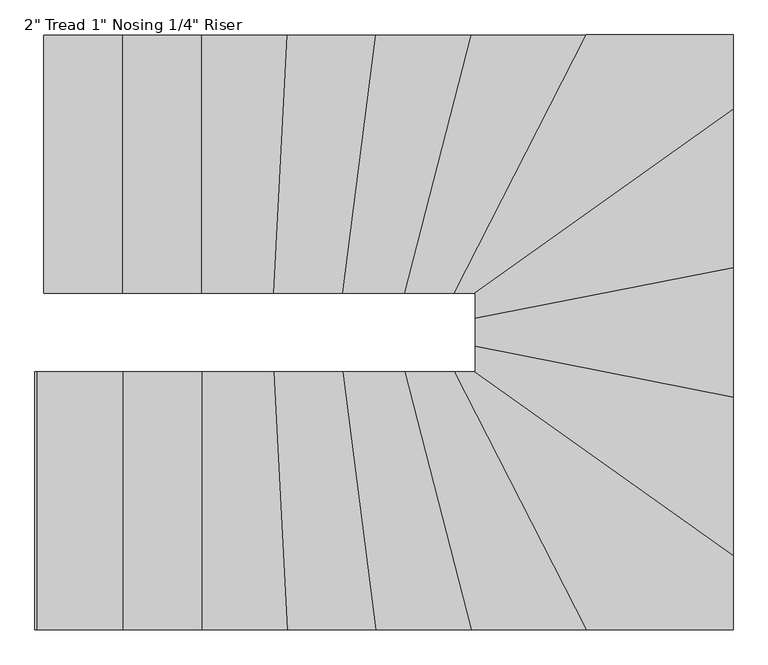
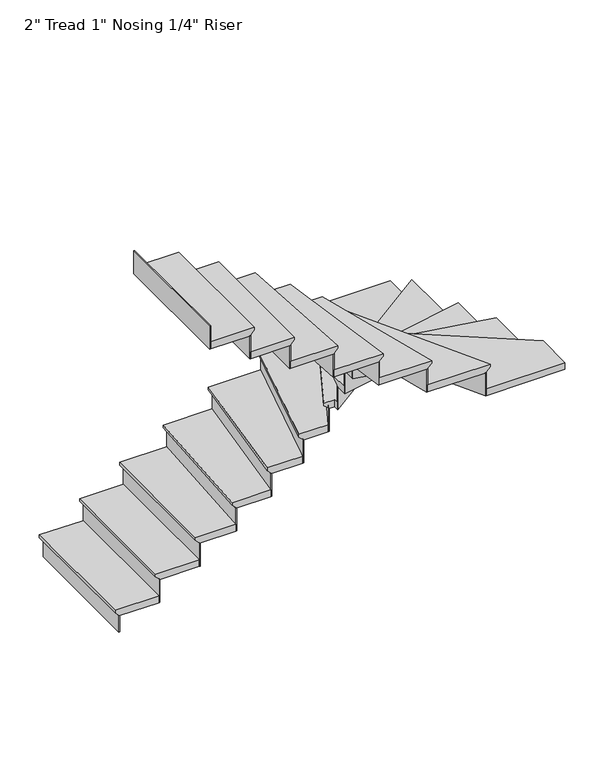
"""IFC4 building model written with IfcOpenShell, lengths in millimetres: stair flight geometry."""

from ifc_helpers import new_model, si_unit, origin, place, context, project, spatial, faceted_brep, source, transform, mapped, element, save


def stair_flight_9e462077(model_context):
    return source(origin(), model_context, "Body", "Brep", [
        faceted_brep([(1342.8282136, -2159.7365003, 9751.4833333), (1342.8282136, -2159.7365003, 9770.5333333), (1342.8282136, -1245.3365003, 9770.5333333), (1342.8282136, -1245.3365003, 9751.4833333), (1368.2282136, -2159.7365003, 9726.0833333), (1368.2282136, -1245.3365003, 9726.0833333), (1647.6282136, -2159.7365003, 9770.5333333), (1647.6282136, -1245.3365003, 9770.5333333), (1368.2282136, -1245.3365003, 9719.7333333), (1647.6282136, -1245.3365003, 9719.7333333), (1647.6282136, -2159.7365003, 9719.7333333), (1368.2282136, -2159.7365003, 9719.7333333)], [[[0, 1, 2, 3]], [[4, 0, 3, 5]], [[2, 1, 6, 7]], [[8, 9, 10, 11]], [[2, 7, 9, 8, 5, 3]], [[8, 11, 4, 5]], [[6, 1, 0, 4, 11, 10]], [[7, 6, 10, 9]]]),
        faceted_brep([(1368.2282136, -2159.7365003, 9719.7333333), (1368.2282136, -2159.7365003, 9601.2), (1374.5782136, -2159.7365003, 9601.2), (1374.5782136, -2159.7365003, 9719.7333333), (1368.2282136, -1245.3365003, 9719.7333333), (1374.5782136, -1245.3365003, 9719.7333333), (1374.5782136, -1245.3365003, 9601.2), (1368.2282136, -1245.3365003, 9601.2)], [[[0, 1, 2, 3]], [[4, 5, 6, 7]], [[1, 0, 4, 7]], [[2, 1, 7, 6]], [[3, 2, 6, 5]], [[0, 3, 5, 4]]]),
        faceted_brep([(1647.6282136, -2159.7365003, 9889.0666667), (1647.6282136, -2159.7365003, 9719.7333333), (1653.9782136, -2159.7365003, 9719.7333333), (1653.9782136, -2159.7365003, 9889.0666667), (1647.6282136, -1245.3365003, 9889.0666667), (1653.9782136, -1245.3365003, 9889.0666667), (1653.9782136, -1245.3365003, 9719.7333333), (1647.6282136, -1245.3365003, 9719.7333333)], [[[0, 1, 2, 3]], [[4, 5, 6, 7]], [[1, 0, 4, 7]], [[2, 1, 7, 6]], [[3, 2, 6, 5]], [[0, 3, 5, 4]]]),
        faceted_brep([(1622.2282136, -1245.3365003, 9939.8666667), (1622.2282136, -2159.7365003, 9939.8666667), (1927.0282136, -2159.7365003, 9939.8666667), (1927.0282136, -1245.3365003, 9939.8666667), (1647.6282136, -1245.3365003, 9889.0666667), (1927.0282136, -1245.3365003, 9889.0666667), (1927.0282136, -2159.7365003, 9889.0666667), (1647.6282136, -2159.7365003, 9889.0666667), (1647.6282136, -1245.3365003, 9895.4166667), (1622.2282136, -1245.3365003, 9920.8166667), (1647.6282136, -2159.7365003, 9895.4166667), (1622.2282136, -2159.7365003, 9920.8166667)], [[[0, 1, 2, 3]], [[4, 5, 6, 7]], [[0, 3, 5, 4, 8, 9]], [[4, 7, 10, 8]], [[2, 1, 11, 10, 7, 6]], [[3, 2, 6, 5]], [[11, 1, 0, 9]], [[10, 11, 9, 8]]]),
        faceted_brep([(1927.0282136, -2159.7365003, 10058.4), (1927.0282136, -2159.7365003, 9889.0666667), (1933.3782136, -2159.7365003, 9889.0666667), (1933.3782136, -2159.7365003, 10058.4), (1927.0282136, -1245.3365003, 10058.4), (1933.3782136, -1245.3365003, 10058.4), (1933.3782136, -1245.3365003, 9889.0666667), (1927.0282136, -1245.3365003, 9889.0666667)], [[[0, 1, 2, 3]], [[4, 5, 6, 7]], [[1, 0, 4, 7]], [[2, 1, 7, 6]], [[3, 2, 6, 5]], [[0, 3, 5, 4]]]),
        faceted_brep([(1901.6282136, -1245.3365003, 10109.2), (1901.6282136, -2159.7365003, 10109.2), (2182.6953751, -2159.7365003, 10109.2), (2230.2296455, -1245.3365003, 10109.2), (1927.0282136, -1245.3365003, 10058.4), (2230.2296455, -1245.3365003, 10058.4), (2182.6953751, -2159.7365003, 10058.4), (1927.0282136, -2159.7365003, 10058.4), (1927.0282136, -1245.3365003, 10064.75), (1901.6282136, -1245.3365003, 10090.15), (1927.0282136, -2159.7365003, 10064.75), (1901.6282136, -2159.7365003, 10090.15)], [[[0, 1, 2, 3]], [[4, 5, 6, 7]], [[0, 3, 5, 4, 8, 9]], [[4, 7, 10, 8]], [[2, 1, 11, 10, 7, 6]], [[3, 2, 6, 5]], [[11, 1, 0, 9]], [[10, 11, 9, 8]]]),
        faceted_brep([(2182.6953751, -2159.7365003, 10227.7333333), (2182.6953751, -2159.7365003, 10058.4), (2189.0539493, -2159.7365003, 10058.4), (2189.0539493, -2159.7365003, 10227.7333333), (2230.2296455, -1245.3365003, 10227.7333333), (2236.5882197, -1245.3365003, 10227.7333333), (2236.5882197, -1245.3365003, 10058.4), (2230.2296455, -1245.3365003, 10058.4)], [[[0, 1, 2, 3]], [[4, 5, 6, 7]], [[1, 0, 4, 7]], [[2, 1, 7, 6]], [[3, 2, 6, 5]], [[0, 3, 5, 4]]]),
        faceted_brep([(2204.7953488, -1245.3365003, 10278.5333333), (2157.2610784, -2159.7365003, 10278.5333333), (2426.8620749, -2159.7365003, 10278.5333333), (2545.2181266, -1245.3365003, 10278.5333333), (2230.2296455, -1245.3365003, 10227.7333333), (2545.2181266, -1245.3365003, 10227.7333333), (2426.8620749, -2159.7365003, 10227.7333333), (2182.6953751, -2159.7365003, 10227.7333333), (2230.2296455, -1245.3365003, 10234.0833333), (2204.7953488, -1245.3365003, 10259.4833333), (2182.6953751, -2159.7365003, 10234.0833333), (2157.2610784, -2159.7365003, 10259.4833333)], [[[0, 1, 2, 3]], [[4, 5, 6, 7]], [[0, 3, 5, 4, 8, 9]], [[4, 7, 10, 8]], [[2, 1, 11, 10, 7, 6]], [[3, 2, 6, 5]], [[11, 1, 0, 9]], [[10, 11, 9, 8]]]),
        faceted_brep([(2426.8620749, -2159.7365003, 10397.0666667), (2426.8620749, -2159.7365003, 10227.7333333), (2433.2650467, -2159.7365003, 10227.7333333), (2433.2650467, -2159.7365003, 10397.0666667), (2545.2181266, -1245.3365003, 10397.0666667), (2551.6210984, -1245.3365003, 10397.0666667), (2551.6210984, -1245.3365003, 10227.7333333), (2545.2181266, -1245.3365003, 10227.7333333)], [[[0, 1, 2, 3]], [[4, 5, 6, 7]], [[1, 0, 4, 7]], [[2, 1, 7, 6]], [[3, 2, 6, 5]], [[0, 3, 5, 4]]]),
        faceted_brep([(2519.6062395, -1245.3365003, 10447.8666667), (2401.2501878, -2159.7365003, 10447.8666667), (2648.4892974, -2159.7365003, 10447.8666667), (2883.6197448, -1245.3365003, 10447.8666667), (2545.2181266, -1245.3365003, 10397.0666667), (2883.6197448, -1245.3365003, 10397.0666667), (2648.4892974, -2159.7365003, 10397.0666667), (2426.8620749, -2159.7365003, 10397.0666667), (2545.2181266, -1245.3365003, 10403.4166667), (2519.6062395, -1245.3365003, 10428.8166667), (2426.8620749, -2159.7365003, 10403.4166667), (2401.2501878, -2159.7365003, 10428.8166667)], [[[0, 1, 2, 3]], [[4, 5, 6, 7]], [[0, 3, 5, 4, 8, 9]], [[4, 7, 10, 8]], [[2, 1, 11, 10, 7, 6]], [[3, 2, 6, 5]], [[11, 1, 0, 9]], [[10, 11, 9, 8]]]),
        faceted_brep([(2648.4892974, -2159.7365003, 10566.4), (2648.4892974, -2159.7365003, 10397.0666667), (2655.0458743, -2159.7365003, 10397.0666667), (2655.0458743, -2159.7365003, 10566.4), (2883.6197448, -1245.3365003, 10566.4), (2890.1763217, -1245.3365003, 10566.4), (2890.1763217, -1245.3365003, 10397.0666667), (2883.6197448, -1245.3365003, 10397.0666667)], [[[0, 1, 2, 3]], [[4, 5, 6, 7]], [[1, 0, 4, 7]], [[2, 1, 7, 6]], [[3, 2, 6, 5]], [[0, 3, 5, 4]]]),
        faceted_brep([(2857.3934373, -1245.3365003, 10617.2), (2622.2629899, -2159.7365003, 10617.2), (2824.8359335, -2159.7365003, 10617.2), (3293.6605548, -1245.3365003, 10617.2), (2883.6197448, -1245.3365003, 10566.4), (3293.6605548, -1245.3365003, 10566.4), (2824.8359335, -2159.7365003, 10566.4), (2648.4892974, -2159.7365003, 10566.4), (2883.6197448, -1245.3365003, 10572.75), (2857.3934373, -1245.3365003, 10598.15), (2648.4892974, -2159.7365003, 10572.75), (2622.2629899, -2159.7365003, 10598.15)], [[[0, 1, 2, 3]], [[4, 5, 6, 7]], [[0, 3, 5, 4, 8, 9]], [[4, 7, 10, 8]], [[2, 1, 11, 10, 7, 6]], [[3, 2, 6, 5]], [[11, 1, 0, 9]], [[10, 11, 9, 8]]]),
        faceted_brep([(2824.8359335, -2159.7365003, 10735.7333333), (2824.8359335, -2159.7365003, 10566.4), (2831.9719166, -2159.7365003, 10566.4), (2831.9719166, -2159.7365003, 10735.7333333), (3293.6605548, -1245.3365003, 10735.7333333), (3300.7965379, -1245.3365003, 10735.7333333), (3300.7965379, -1245.3365003, 10566.4), (3293.6605548, -1245.3365003, 10566.4)], [[[0, 1, 2, 3]], [[4, 5, 6, 7]], [[1, 0, 4, 7]], [[2, 1, 7, 6]], [[3, 2, 6, 5]], [[0, 3, 5, 4]]]),
        faceted_brep([(3784.9599055, -1539.017634, 10786.5333333), (3784.9599055, -1245.3365003, 10786.5333333), (3265.1166223, -1245.3365003, 10786.5333333), (2796.2920009, -2159.7365003, 10786.5333333), (2870.5599055, -2159.7365003, 10786.5333333), (2870.5599055, -2189.2915832, 10786.5333333), (3784.9599055, -1245.3365003, 10735.7333333), (3784.9599055, -1539.017634, 10735.7333333), (2870.5599055, -2189.2915832, 10735.7333333), (2870.5599055, -2159.7365003, 10735.7333333), (2824.8359335, -2159.7365003, 10735.7333333), (3293.6605548, -1245.3365003, 10735.7333333), (3293.6605548, -1245.3365003, 10742.0833333), (3265.1166223, -1245.3365003, 10767.4833333), (2824.8359335, -2159.7365003, 10742.0833333), (2796.2920009, -2159.7365003, 10767.4833333)], [[[0, 1, 2, 3, 4, 5]], [[6, 7, 8, 9, 10, 11]], [[1, 0, 7, 6]], [[2, 1, 6, 11, 12, 13]], [[11, 10, 14, 12]], [[4, 3, 15, 14, 10, 9]], [[5, 4, 9, 8]], [[0, 5, 8, 7]], [[15, 3, 2, 13]], [[14, 15, 13, 12]]]),
        faceted_brep([(2870.5599055, -2189.2915832, 10905.0666667), (2870.5599055, -2189.2915832, 10735.7333333), (2870.5599055, -2197.083558, 10735.7333333), (2870.5599055, -2197.083558, 10905.0666667), (3784.9599055, -1539.017634, 10905.0666667), (3784.9599055, -1546.8096088, 10905.0666667), (3784.9599055, -1546.8096088, 10735.7333333), (3784.9599055, -1539.017634, 10735.7333333)], [[[0, 1, 2, 3]], [[4, 5, 6, 7]], [[1, 0, 4, 7]], [[2, 1, 7, 6]], [[3, 2, 6, 5]], [[0, 3, 5, 4]]]),
        faceted_brep([(3784.9599055, -1507.8497349, 10955.8666667), (2870.5599055, -2158.123684, 10955.8666667), (2870.5599055, -2275.7456703, 10955.8666667), (3784.9599055, -2095.5048139, 10955.8666667), (3784.9599055, -1539.017634, 10905.0666667), (3784.9599055, -2095.5048139, 10905.0666667), (2870.5599055, -2275.7456703, 10905.0666667), (2870.5599055, -2189.2915832, 10905.0666667), (3784.9599055, -1539.017634, 10911.4166667), (3784.9599055, -1507.8497349, 10936.8166667), (2870.5599055, -2189.2915832, 10911.4166667), (2870.5599055, -2158.123684, 10936.8166667)], [[[0, 1, 2, 3]], [[4, 5, 6, 7]], [[0, 3, 5, 4, 8, 9]], [[4, 7, 10, 8]], [[2, 1, 11, 10, 7, 6]], [[3, 2, 6, 5]], [[11, 1, 0, 9]], [[10, 11, 9, 8]]]),
        faceted_brep([(2870.5599055, -2275.7456703, 11074.4), (2870.5599055, -2275.7456703, 10905.0666667), (2870.5599055, -2282.2178557, 10905.0666667), (2870.5599055, -2282.2178557, 11074.4), (3784.9599055, -2095.5048139, 11074.4), (3784.9599055, -2101.9769994, 11074.4), (3784.9599055, -2101.9769994, 10905.0666667), (3784.9599055, -2095.5048139, 10905.0666667)], [[[0, 1, 2, 3]], [[4, 5, 6, 7]], [[1, 0, 4, 7]], [[2, 1, 7, 6]], [[3, 2, 6, 5]], [[0, 3, 5, 4]]]),
        faceted_brep([(3784.9599055, -2069.6160722, 11125.2), (2870.5599055, -2249.8569285, 11125.2), (2870.5599055, -2374.9048139, 11125.2), (3784.9599055, -2555.1456703, 11125.2), (3784.9599055, -2095.5048139, 11074.4), (3784.9599055, -2555.1456703, 11074.4), (2870.5599055, -2374.9048139, 11074.4), (2870.5599055, -2275.7456703, 11074.4), (3784.9599055, -2095.5048139, 11080.75), (3784.9599055, -2069.6160722, 11106.15), (2870.5599055, -2275.7456703, 11080.75), (2870.5599055, -2249.8569285, 11106.15)], [[[0, 1, 2, 3]], [[4, 5, 6, 7]], [[0, 3, 5, 4, 8, 9]], [[4, 7, 10, 8]], [[2, 1, 11, 10, 7, 6]], [[3, 2, 6, 5]], [[11, 1, 0, 9]], [[10, 11, 9, 8]]]),
        faceted_brep([(2870.5599055, -2374.9048139, 11243.7333333), (2870.5599055, -2374.9048139, 11074.4), (2870.5599055, -2381.3769994, 11074.4), (2870.5599055, -2381.3769994, 11243.7333333), (3784.9599055, -2555.1456703, 11243.7333333), (3784.9599055, -2561.6178557, 11243.7333333), (3784.9599055, -2561.6178557, 11074.4), (3784.9599055, -2555.1456703, 11074.4)], [[[0, 1, 2, 3]], [[4, 5, 6, 7]], [[1, 0, 4, 7]], [[2, 1, 7, 6]], [[3, 2, 6, 5]], [[0, 3, 5, 4]]]),
        faceted_brep([(3784.9599055, -2529.2569285, 11294.5333333), (2870.5599055, -2349.0160722, 11294.5333333), (2870.5599055, -2439.1365003, 11294.5333333), (2824.464431, -2439.1365003, 11294.5333333), (3784.9599055, -3122.191165, 11294.5333333), (3784.9599055, -2555.1456703, 11243.7333333), (3784.9599055, -3122.191165, 11243.7333333), (2824.464431, -2439.1365003, 11243.7333333), (2870.5599055, -2439.1365003, 11243.7333333), (2870.5599055, -2374.9048139, 11243.7333333), (3784.9599055, -2555.1456703, 11250.0833333), (3784.9599055, -2529.2569285, 11275.4833333), (2870.5599055, -2374.9048139, 11250.0833333), (2870.5599055, -2349.0160722, 11275.4833333)], [[[0, 1, 2, 3, 4]], [[5, 6, 7, 8, 9]], [[0, 4, 6, 5, 10, 11]], [[5, 9, 12, 10]], [[2, 1, 13, 12, 9, 8]], [[3, 2, 8, 7]], [[4, 3, 7, 6]], [[13, 1, 0, 11]], [[12, 13, 11, 10]]]),
        faceted_brep([(2824.464431, -2439.1365003, 11413.0666667), (2824.464431, -2439.1365003, 11243.7333333), (2813.5075385, -2439.1365003, 11243.7333333), (2813.5075385, -2439.1365003, 11413.0666667), (3784.9599055, -3122.191165, 11413.0666667), (3784.9599055, -3129.9831398, 11413.0666667), (3784.9599055, -3129.9831398, 11243.7333333), (3784.9599055, -3122.191165, 11243.7333333)], [[[0, 1, 2, 3]], [[4, 5, 6, 7]], [[1, 0, 4, 7]], [[2, 1, 7, 6]], [[3, 2, 6, 5]], [[0, 3, 5, 4]]]),
        faceted_brep([(3236.5726897, -3353.5365003, 11463.8666667), (3784.9599055, -3353.5365003, 11463.8666667), (3784.9599055, -3091.0232658, 11463.8666667), (2868.2920009, -2439.1365003, 11463.8666667), (2767.7480684, -2439.1365003, 11463.8666667), (3784.9599055, -3353.5365003, 11413.0666667), (3236.5726897, -3353.5365003, 11413.0666667), (2767.7480684, -2439.1365003, 11413.0666667), (2824.464431, -2439.1365003, 11413.0666667), (3784.9599055, -3122.191165, 11413.0666667), (3784.9599055, -3122.191165, 11419.4166667), (3784.9599055, -3091.0232658, 11444.8166667), (2824.464431, -2439.1365003, 11419.4166667), (2868.2920009, -2439.1365003, 11444.8166667)], [[[0, 1, 2, 3, 4]], [[5, 6, 7, 8, 9]], [[1, 0, 6, 5]], [[2, 1, 5, 9, 10, 11]], [[9, 8, 12, 10]], [[4, 3, 13, 12, 8, 7]], [[0, 4, 7, 6]], [[13, 3, 2, 11]], [[12, 13, 11, 10]]]),
        faceted_brep([(2767.7480684, -2439.1365003, 11582.4), (2767.7480684, -2439.1365003, 11413.0666667), (2760.6120853, -2439.1365003, 11413.0666667), (2760.6120853, -2439.1365003, 11582.4), (3236.5726897, -3353.5365003, 11582.4), (3229.4367066, -3353.5365003, 11582.4), (3229.4367066, -3353.5365003, 11413.0666667), (3236.5726897, -3353.5365003, 11413.0666667)], [[[0, 1, 2, 3]], [[4, 5, 6, 7]], [[1, 0, 4, 7]], [[2, 1, 7, 6]], [[3, 2, 6, 5]], [[0, 3, 5, 4]]]),
        faceted_brep([(3265.1166223, -3353.5365003, 11633.2), (2796.2920009, -2439.1365003, 11633.2), (2596.0366825, -2439.1365003, 11633.2), (2831.1671299, -3353.5365003, 11633.2), (3236.5726897, -3353.5365003, 11582.4), (2831.1671299, -3353.5365003, 11582.4), (2596.0366825, -2439.1365003, 11582.4), (2767.7480684, -2439.1365003, 11582.4), (3236.5726897, -3353.5365003, 11588.75), (3265.1166223, -3353.5365003, 11614.15), (2767.7480684, -2439.1365003, 11588.75), (2796.2920009, -2439.1365003, 11614.15)], [[[0, 1, 2, 3]], [[4, 5, 6, 7]], [[0, 3, 5, 4, 8, 9]], [[4, 7, 10, 8]], [[2, 1, 11, 10, 7, 6]], [[3, 2, 6, 5]], [[11, 1, 0, 9]], [[10, 11, 9, 8]]]),
        faceted_brep([(2596.0366825, -2439.1365003, 11751.7333333), (2596.0366825, -2439.1365003, 11582.4), (2589.4801056, -2439.1365003, 11582.4), (2589.4801056, -2439.1365003, 11751.7333333), (2831.1671299, -3353.5365003, 11751.7333333), (2824.610553, -3353.5365003, 11751.7333333), (2824.610553, -3353.5365003, 11582.4), (2831.1671299, -3353.5365003, 11582.4)], [[[0, 1, 2, 3]], [[4, 5, 6, 7]], [[1, 0, 4, 7]], [[2, 1, 7, 6]], [[3, 2, 6, 5]], [[0, 3, 5, 4]]]),
        faceted_brep([(2857.3934373, -3353.5365003, 11802.5333333), (2622.2629899, -2439.1365003, 11802.5333333), (2375.6383007, -2439.1365003, 11802.5333333), (2493.9943524, -3353.5365003, 11802.5333333), (2831.1671299, -3353.5365003, 11751.7333333), (2493.9943524, -3353.5365003, 11751.7333333), (2375.6383007, -2439.1365003, 11751.7333333), (2596.0366825, -2439.1365003, 11751.7333333), (2831.1671299, -3353.5365003, 11758.0833333), (2857.3934373, -3353.5365003, 11783.4833333), (2596.0366825, -2439.1365003, 11758.0833333), (2622.2629899, -2439.1365003, 11783.4833333)], [[[0, 1, 2, 3]], [[4, 5, 6, 7]], [[0, 3, 5, 4, 8, 9]], [[4, 7, 10, 8]], [[2, 1, 11, 10, 7, 6]], [[3, 2, 6, 5]], [[11, 1, 0, 9]], [[10, 11, 9, 8]]]),
        faceted_brep([(2375.6383007, -2439.1365003, 11921.0666667), (2375.6383007, -2439.1365003, 11751.7333333), (2369.2353289, -2439.1365003, 11751.7333333), (2369.2353289, -2439.1365003, 11921.0666667), (2493.9943524, -3353.5365003, 11921.0666667), (2487.5913806, -3353.5365003, 11921.0666667), (2487.5913806, -3353.5365003, 11751.7333333), (2493.9943524, -3353.5365003, 11751.7333333)], [[[0, 1, 2, 3]], [[4, 5, 6, 7]], [[1, 0, 4, 7]], [[2, 1, 7, 6]], [[3, 2, 6, 5]], [[0, 3, 5, 4]]]),
        faceted_brep([(2519.6062395, -3353.5365003, 11971.8666667), (2401.2501878, -2439.1365003, 11971.8666667), (2131.8267818, -2439.1365003, 11971.8666667), (2179.3610522, -3353.5365003, 11971.8666667), (2493.9943524, -3353.5365003, 11921.0666667), (2179.3610522, -3353.5365003, 11921.0666667), (2131.8267818, -2439.1365003, 11921.0666667), (2375.6383007, -2439.1365003, 11921.0666667), (2493.9943524, -3353.5365003, 11927.4166667), (2519.6062395, -3353.5365003, 11952.8166667), (2375.6383007, -2439.1365003, 11927.4166667), (2401.2501878, -2439.1365003, 11952.8166667)], [[[0, 1, 2, 3]], [[4, 5, 6, 7]], [[0, 3, 5, 4, 8, 9]], [[4, 7, 10, 8]], [[2, 1, 11, 10, 7, 6]], [[3, 2, 6, 5]], [[11, 1, 0, 9]], [[10, 11, 9, 8]]]),
        faceted_brep([(2131.8267818, -2439.1365003, 12090.4), (2131.8267818, -2439.1365003, 11921.0666667), (2125.4682076, -2439.1365003, 11921.0666667), (2125.4682076, -2439.1365003, 12090.4), (2179.3610522, -3353.5365003, 12090.4), (2173.002478, -3353.5365003, 12090.4), (2173.002478, -3353.5365003, 11921.0666667), (2179.3610522, -3353.5365003, 11921.0666667)], [[[0, 1, 2, 3]], [[4, 5, 6, 7]], [[1, 0, 4, 7]], [[2, 1, 7, 6]], [[3, 2, 6, 5]], [[0, 3, 5, 4]]]),
        faceted_brep([(2204.7953488, -3353.5365003, 12141.2), (2157.2610784, -2439.1365003, 12141.2), (1876.2282136, -2439.1365003, 12141.2), (1876.2282136, -3353.5365003, 12141.2), (2179.3610522, -3353.5365003, 12090.4), (1876.2282136, -3353.5365003, 12090.4), (1876.2282136, -2439.1365003, 12090.4), (2131.8267818, -2439.1365003, 12090.4), (2179.3610522, -3353.5365003, 12096.75), (2204.7953488, -3353.5365003, 12122.15), (2131.8267818, -2439.1365003, 12096.75), (2157.2610784, -2439.1365003, 12122.15)], [[[0, 1, 2, 3]], [[4, 5, 6, 7]], [[0, 3, 5, 4, 8, 9]], [[4, 7, 10, 8]], [[2, 1, 11, 10, 7, 6]], [[3, 2, 6, 5]], [[11, 1, 0, 9]], [[10, 11, 9, 8]]]),
        faceted_brep([(1876.2282136, -2439.1365003, 12259.7333333), (1876.2282136, -2439.1365003, 12090.4), (1869.8782136, -2439.1365003, 12090.4), (1869.8782136, -2439.1365003, 12259.7333333), (1876.2282136, -3353.5365003, 12259.7333333), (1869.8782136, -3353.5365003, 12259.7333333), (1869.8782136, -3353.5365003, 12090.4), (1876.2282136, -3353.5365003, 12090.4)], [[[0, 1, 2, 3]], [[4, 5, 6, 7]], [[1, 0, 4, 7]], [[2, 1, 7, 6]], [[3, 2, 6, 5]], [[0, 3, 5, 4]]]),
        faceted_brep([(1901.6282136, -3353.5365003, 12310.5333333), (1901.6282136, -2439.1365003, 12310.5333333), (1596.8282136, -2439.1365003, 12310.5333333), (1596.8282136, -3353.5365003, 12310.5333333), (1876.2282136, -3353.5365003, 12259.7333333), (1596.8282136, -3353.5365003, 12259.7333333), (1596.8282136, -2439.1365003, 12259.7333333), (1876.2282136, -2439.1365003, 12259.7333333), (1876.2282136, -3353.5365003, 12266.0833333), (1901.6282136, -3353.5365003, 12291.4833333), (1876.2282136, -2439.1365003, 12266.0833333), (1901.6282136, -2439.1365003, 12291.4833333)], [[[0, 1, 2, 3]], [[4, 5, 6, 7]], [[0, 3, 5, 4, 8, 9]], [[4, 7, 10, 8]], [[2, 1, 11, 10, 7, 6]], [[3, 2, 6, 5]], [[11, 1, 0, 9]], [[10, 11, 9, 8]]]),
        faceted_brep([(1596.8282136, -2439.1365003, 12429.0666667), (1596.8282136, -2439.1365003, 12259.7333333), (1590.4782136, -2439.1365003, 12259.7333333), (1590.4782136, -2439.1365003, 12429.0666667), (1596.8282136, -3353.5365003, 12429.0666667), (1590.4782136, -3353.5365003, 12429.0666667), (1590.4782136, -3353.5365003, 12259.7333333), (1596.8282136, -3353.5365003, 12259.7333333)], [[[0, 1, 2, 3]], [[4, 5, 6, 7]], [[1, 0, 4, 7]], [[2, 1, 7, 6]], [[3, 2, 6, 5]], [[0, 3, 5, 4]]]),
        faceted_brep([(1317.4282136, -2439.1365003, 12598.4), (1317.4282136, -2439.1365003, 12429.0666667), (1311.0782136, -2439.1365003, 12429.0666667), (1311.0782136, -2439.1365003, 12598.4), (1317.4282136, -3353.5365003, 12598.4), (1311.0782136, -3353.5365003, 12598.4), (1311.0782136, -3353.5365003, 12429.0666667), (1317.4282136, -3353.5365003, 12429.0666667)], [[[0, 1, 2, 3]], [[4, 5, 6, 7]], [[1, 0, 4, 7]], [[2, 1, 7, 6]], [[3, 2, 6, 5]], [[0, 3, 5, 4]]]),
        faceted_brep([(1622.2282136, -3353.5365003, 12479.8666667), (1622.2282136, -2439.1365003, 12479.8666667), (1317.4282136, -2439.1365003, 12479.8666667), (1317.4282136, -3353.5365003, 12479.8666667), (1596.8282136, -3353.5365003, 12429.0666667), (1317.4282136, -3353.5365003, 12429.0666667), (1317.4282136, -2439.1365003, 12429.0666667), (1596.8282136, -2439.1365003, 12429.0666667), (1596.8282136, -3353.5365003, 12435.4166667), (1622.2282136, -3353.5365003, 12460.8166667), (1596.8282136, -2439.1365003, 12435.4166667), (1622.2282136, -2439.1365003, 12460.8166667)], [[[0, 1, 2, 3]], [[4, 5, 6, 7]], [[0, 3, 5, 4, 8, 9]], [[4, 7, 10, 8]], [[2, 1, 11, 10, 7, 6]], [[3, 2, 6, 5]], [[11, 1, 0, 9]], [[10, 11, 9, 8]]]),
    ])


if __name__ == "__main__":
    model = new_model("IFC4")
    model_context = context("Model", 3, world=origin())
    ifc_project = project(units=[si_unit("LENGTHUNIT", "METRE", prefix="MILLI")], contexts=[model_context])
    site = spatial("IfcSite", under=ifc_project)
    building = spatial("IfcBuilding", under=site)
    placement = place(None, origin())
    stair_flight_shape = stair_flight_9e462077(model_context)
    element("IfcStairFlight", 1, ObjectType="2\" Tread 1\" Nosing 1/4\" Riser", at=placement, inside=building, context=model_context, shape_type="MappedRepresentation", body=[
        mapped(stair_flight_shape, transform((0.0, 0.0, 0.0), x_axis=(1.0, 0.0, 0.0), y_axis=(0.0, 1.0, 0.0), z_axis=(0.0, 0.0, 1.0))),
    ])
    save(model, "model.ifc")
